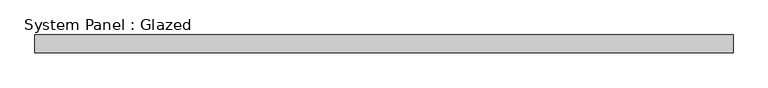
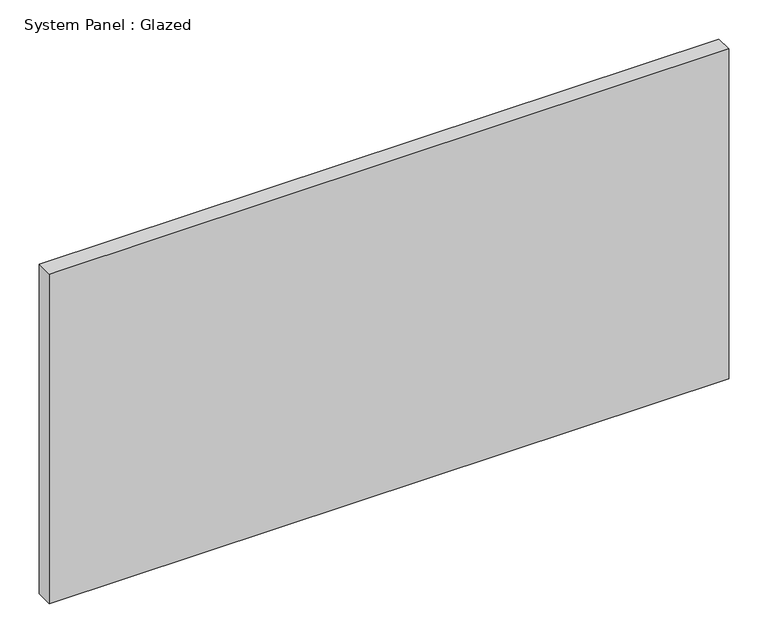
"""IFC4 building model written with IfcOpenShell, lengths in millimetres: plate geometry, System Panel : Glazed."""

from ifc_helpers import new_model, si_unit, origin, origin_with_axes, place, context, project, spatial, polyline, outline, extrude, source, transform, mapped, element, save


def system_panel_glazed_ff9ba4bf(model_context):
    return source(origin(), model_context, "Body", "SweptSolid", [
        extrude(outline(polyline([(501.6499999, 19.05), (-501.6499999, 19.05), (-501.6499999, 44.45), (501.6499999, 44.45), (501.6499999, 19.05)])), origin_with_axes(), (0.0, 0.0, 1.0), 514.35),
    ])


if __name__ == "__main__":
    model = new_model("IFC4")
    model_context = context("Model", 3, world=origin())
    ifc_project = project(units=[si_unit("LENGTHUNIT", "METRE", prefix="MILLI")], contexts=[model_context])
    site = spatial("IfcSite", under=ifc_project)
    building = spatial("IfcBuilding", under=site)
    placement = place(None, origin())
    system_panel_glazed_shape = system_panel_glazed_ff9ba4bf(model_context)
    element("IfcPlate", 1, ObjectType="System Panel : Glazed", at=placement, inside=building, context=model_context, shape_type="MappedRepresentation", body=[
        mapped(system_panel_glazed_shape, transform((0.0, 0.0, 0.0), x_axis=(1.0, 0.0, 0.0), y_axis=(0.0, 1.0, 0.0), z_axis=(0.0, 0.0, 1.0))),
    ])
    save(model, "model.ifc")

# Revit data of these elements
# Type "System Panel : Glazed"
#   Construction Type Id = "GSP4R"
#   Analytic Construction = "1/8 in Pilkington single glazing"
#   Visual Light Transmittance = 0.9
#   Solar Heat Gain Coefficient = 0.86
#   Heat Transfer Coefficient (U) = 1.18115 BTU/(h·ft²·°F)
#   Define Thermal Properties by = 1
# Element 1 (IfcPlate, "System Panel : Glazed")
#   Materials on its faces: "Glass"
# Materials
#   "Glass": class "Glass", colour RGB 0 128 192, transparency 0.75, Description = "Soda Lime Glass", Cost = 0
